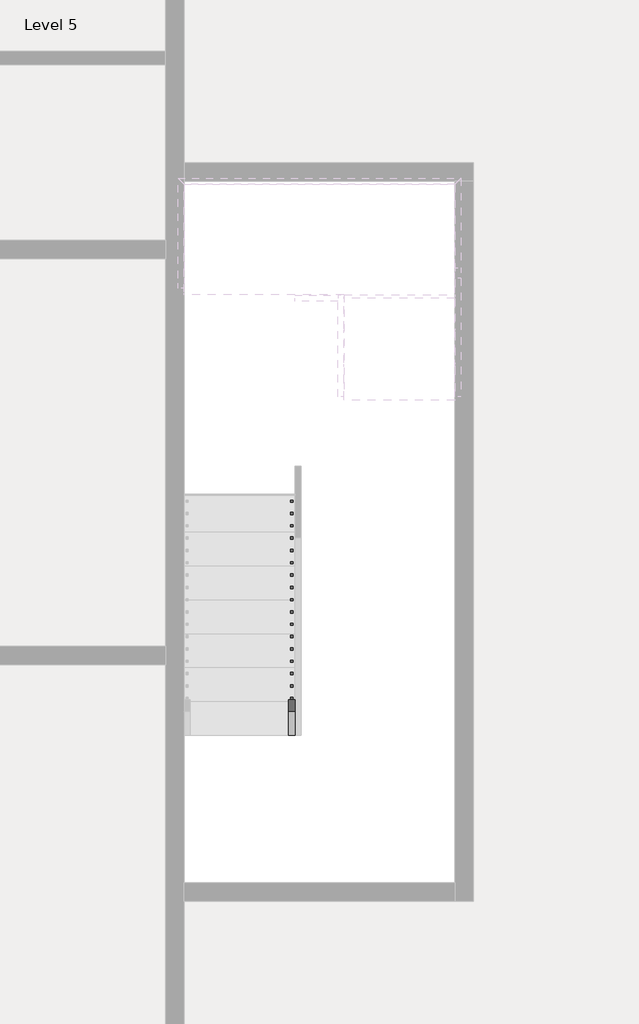
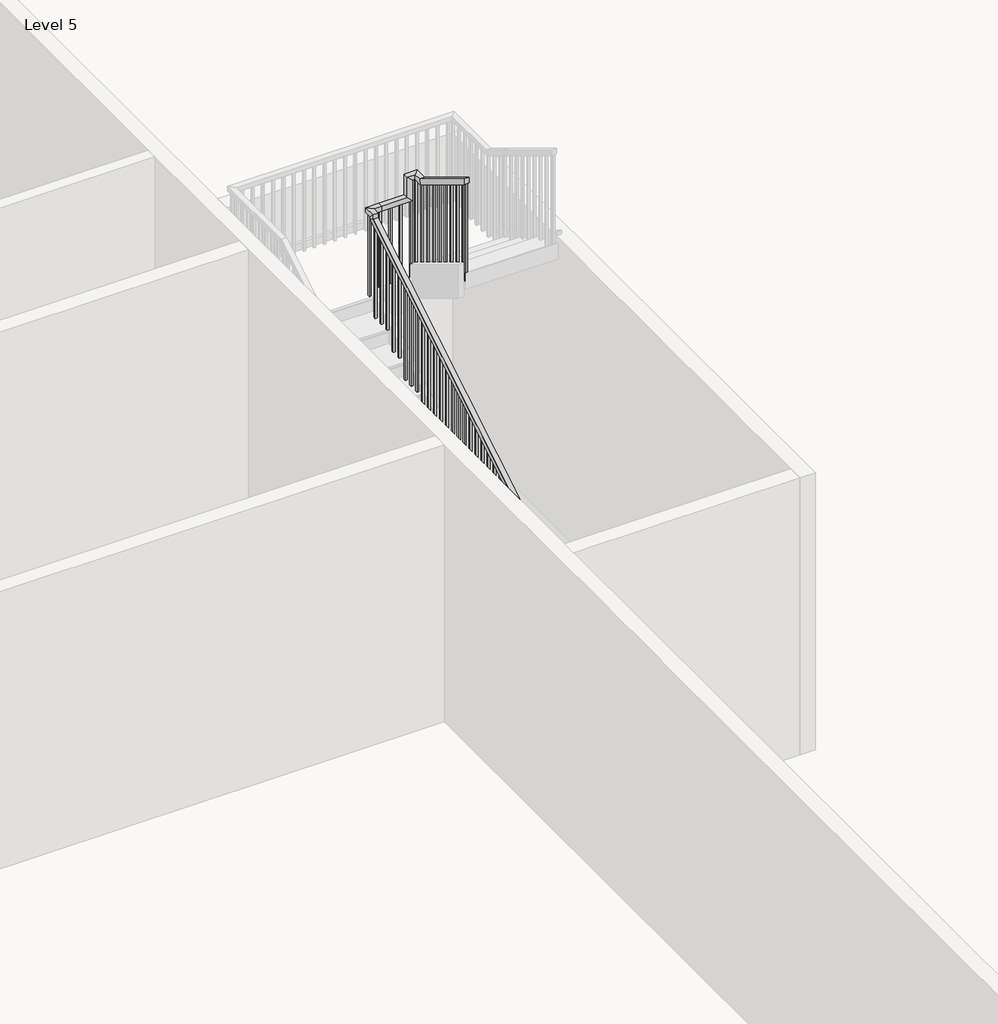
# One storey, part 5 of 8: 1 railing.
"""IFC4 building model written with IfcOpenShell, lengths in millimetres."""

from ifc_helpers import new_model, si_unit, frame, origin, place, context, project, spatial, polyline, outline, extrude, faceted_brep, element, save

model = new_model("IFC4")

# Units and contexts
model_context = context("Model", 3, world=origin())
ifc_project = project(units=[si_unit("LENGTHUNIT", "METRE", prefix="MILLI")], contexts=[model_context])

# Site, building, storey
site = spatial("IfcSite", under=ifc_project)
building = spatial("IfcBuilding", under=site)
storey = spatial("IfcBuildingStorey", under=building, Name="Level 5", Elevation=37426.6172466)

# Railing
placement = place(None, origin())
element("IfcRailing", 1, ObjectType="Handrail - Rectangular", at=placement, inside=storey, context=model_context, shape_type="SolidModel", body=[
    faceted_brep([(-2753.8415084, -23154.3851539, 38510.3505799), (-2753.8415084, -23154.3851539, 38450.9491197), (-2703.0415084, -23154.3851539, 38450.9491197), (-2703.0415084, -23154.3851539, 38510.3505799), (-2753.8415084, -19598.3851539, 40665.5020951), (-2753.8415084, -19547.5851539, 40636.8885136), (-2703.0415084, -19547.5851539, 40636.8885136), (-2703.0415084, -19598.3851539, 40665.5020951), (-2753.8415084, -19598.3851539, 40711.6839133), (-2753.8415084, -19547.5851539, 40660.8839133), (-2703.0415084, -19547.5851539, 40660.8839133), (-2703.0415084, -19598.3851539, 40711.6839133), (-2753.8415084, -19471.3851539, 40711.6839133), (-2753.8415084, -19471.3851539, 40660.8839133), (-2703.0415084, -19522.1851539, 40660.8839133), (-2703.0415084, -19522.1851539, 40711.6839133), (-2626.8415084, -19471.3851539, 40711.6839133), (-2626.8415084, -19471.3851539, 40660.8839133), (-2626.8415084, -19522.1851539, 40660.8839133), (-2626.8415084, -19522.1851539, 40711.6839133), (-2372.8415084, -19471.3851539, 40711.6839133), (-2322.0415084, -19471.3851539, 40660.8839133), (-2322.0415084, -19522.1851539, 40660.8839133), (-2372.8415084, -19522.1851539, 40711.6839133), (-2372.8415084, -19471.3851539, 40927.1990648), (-2322.0415084, -19471.3851539, 40876.3990648), (-2322.0415084, -19522.1851539, 40876.3990648), (-2372.8415084, -19522.1851539, 40927.1990648), (-2245.8415084, -19471.3851539, 40927.1990648), (-2245.8415084, -19471.3851539, 40876.3990648), (-2296.6415084, -19522.1851539, 40876.3990648), (-2296.6415084, -19522.1851539, 40927.1990648), (-2245.8415084, -19598.3851539, 40927.1990648), (-2245.8415084, -19612.5775633, 40876.3990648), (-2296.6415084, -19612.5775633, 40876.3990648), (-2296.6415084, -19598.3851539, 40927.1990648), (-2245.8415084, -20360.3851539, 41389.0172466), (-2296.6415084, -20360.3851539, 41389.0172466), (-2296.6415084, -20360.3851539, 41329.6157863), (-2245.8415084, -20360.3851539, 41329.6157863)], [[[0, 1, 2, 3]], [[1, 0, 4, 5]], [[2, 1, 5, 6]], [[3, 2, 6, 7]], [[0, 3, 7, 4]], [[5, 4, 8, 9]], [[6, 5, 9, 10]], [[7, 6, 10, 11]], [[4, 7, 11, 8]], [[9, 8, 12, 13]], [[10, 9, 13, 14]], [[11, 10, 14, 15]], [[8, 11, 15, 12]], [[13, 12, 16, 17]], [[14, 13, 17, 18]], [[15, 14, 18, 19]], [[12, 15, 19, 16]], [[17, 16, 20, 21]], [[18, 17, 21, 22]], [[19, 18, 22, 23]], [[16, 19, 23, 20]], [[21, 20, 24, 25]], [[22, 21, 25, 26]], [[23, 22, 26, 27]], [[20, 23, 27, 24]], [[25, 24, 28, 29]], [[26, 25, 29, 30]], [[27, 26, 30, 31]], [[24, 27, 31, 28]], [[29, 28, 32, 33]], [[30, 29, 33, 34]], [[31, 30, 34, 35]], [[28, 31, 35, 32]], [[36, 37, 38, 39]], [[33, 32, 36, 39]], [[34, 33, 39, 38]], [[35, 34, 38, 37]], [[32, 35, 37, 36]]]),
    extrude(outline(polyline([(-20319.1101539, 41304.6006348), (-20300.0601539, 41293.0551803), (-20300.0601539, 40305.2839133), (-20319.1101539, 40305.2839133), (-20319.1101539, 41304.6006348)])), frame((-2280.7665084, 0.0, 0.0), z_axis=(1.0, 0.0, 0.0), x_axis=(0.0, 1.0, 0.0)), (0.0, 0.0, 1.0), 19.05),
    extrude(outline(polyline([(-20217.5101539, 41243.0248773), (-20198.4601539, 41231.4794227), (-20198.4601539, 40305.2839133), (-20217.5101539, 40305.2839133), (-20217.5101539, 41243.0248773)])), frame((-2280.7665084, 0.0, 0.0), z_axis=(1.0, 0.0, 0.0), x_axis=(0.0, 1.0, 0.0)), (0.0, 0.0, 1.0), 19.05),
    extrude(outline(polyline([(-20115.9101539, 41181.4491197), (-20096.8601539, 41169.9036651), (-20096.8601539, 40305.2839133), (-20115.9101539, 40305.2839133), (-20115.9101539, 41181.4491197)])), frame((-2280.7665084, 0.0, 0.0), z_axis=(1.0, 0.0, 0.0), x_axis=(0.0, 1.0, 0.0)), (0.0, 0.0, 1.0), 19.05),
    extrude(outline(polyline([(-20014.3101539, 41119.8733621), (-19995.2601539, 41108.3279076), (-19995.2601539, 40135.9505799), (-20014.3101539, 40135.9505799), (-20014.3101539, 41119.8733621)])), frame((-2280.7665084, 0.0, 0.0), z_axis=(1.0, 0.0, 0.0), x_axis=(0.0, 1.0, 0.0)), (0.0, 0.0, 1.0), 19.05),
    extrude(outline(polyline([(-19912.7101539, 41058.2976045), (-19893.6601539, 41046.75215), (-19893.6601539, 40135.9505799), (-19912.7101539, 40135.9505799), (-19912.7101539, 41058.2976045)])), frame((-2280.7665084, 0.0, 0.0), z_axis=(1.0, 0.0, 0.0), x_axis=(0.0, 1.0, 0.0)), (0.0, 0.0, 1.0), 19.05),
    extrude(outline(polyline([(-19811.1101539, 40996.721847), (-19792.0601539, 40985.1763924), (-19792.0601539, 40135.9505799), (-19811.1101539, 40135.9505799), (-19811.1101539, 40996.721847)])), frame((-2280.7665084, 0.0, 0.0), z_axis=(1.0, 0.0, 0.0), x_axis=(0.0, 1.0, 0.0)), (0.0, 0.0, 1.0), 19.05),
    extrude(outline(polyline([(-19709.5101539, 40935.1460894), (-19690.4601539, 40923.6006348), (-19690.4601539, 39966.6172466), (-19709.5101539, 39966.6172466), (-19709.5101539, 40935.1460894)])), frame((-2280.7665084, 0.0, 0.0), z_axis=(1.0, 0.0, 0.0), x_axis=(0.0, 1.0, 0.0)), (0.0, 0.0, 1.0), 19.05),
    extrude(outline(polyline([(-19607.9101539, 40873.5703318), (-19588.8601539, 40862.0248773), (-19588.8601539, 39966.6172466), (-19607.9101539, 39966.6172466), (-19607.9101539, 40873.5703318)])), frame((-2280.7665084, 0.0, 0.0), z_axis=(1.0, 0.0, 0.0), x_axis=(0.0, 1.0, 0.0)), (0.0, 0.0, 1.0), 19.05),
    extrude(outline(polyline([(-2331.5665084, -19506.3101539), (-2331.5665084, -19487.2601539), (-2312.5165084, -19487.2601539), (-2312.5165084, -19506.3101539), (-2331.5665084, -19506.3101539)])), frame((0.0, 0.0, 39797.2839133), z_axis=(0.0, 0.0, 1.0), x_axis=(1.0, 0.0, 0.0)), (0.0, 0.0, 1.0), 1079.1151515),
    extrude(outline(polyline([(-2433.1665084, -19506.3101539), (-2433.1665084, -19487.2601539), (-2414.1165084, -19487.2601539), (-2414.1165084, -19506.3101539), (-2433.1665084, -19506.3101539)])), frame((0.0, 0.0, 39797.2839133), z_axis=(0.0, 0.0, 1.0), x_axis=(1.0, 0.0, 0.0)), (0.0, 0.0, 1.0), 863.6),
    extrude(outline(polyline([(-2534.7665084, -19506.3101539), (-2534.7665084, -19487.2601539), (-2515.7165084, -19487.2601539), (-2515.7165084, -19506.3101539), (-2534.7665084, -19506.3101539)])), frame((0.0, 0.0, 39797.2839133), z_axis=(0.0, 0.0, 1.0), x_axis=(1.0, 0.0, 0.0)), (0.0, 0.0, 1.0), 863.6),
    extrude(outline(polyline([(-2636.3665084, -19506.3101539), (-2636.3665084, -19487.2601539), (-2617.3165084, -19487.2601539), (-2617.3165084, -19506.3101539), (-2636.3665084, -19506.3101539)])), frame((0.0, 0.0, 39797.2839133), z_axis=(0.0, 0.0, 1.0), x_axis=(1.0, 0.0, 0.0)), (0.0, 0.0, 1.0), 863.6),
    extrude(outline(polyline([(-19607.9101539, 40600.3279076), (-19588.8601539, 40611.8733621), (-19588.8601539, 39627.9505799), (-19607.9101539, 39627.9505799), (-19607.9101539, 40600.3279076)])), frame((-2737.9665084, 0.0, 0.0), z_axis=(1.0, 0.0, 0.0), x_axis=(0.0, 1.0, 0.0)), (0.0, 0.0, 1.0), 19.05),
    extrude(outline(polyline([(-19709.5101539, 40538.75215), (-19690.4601539, 40550.2976045), (-19690.4601539, 39627.9505799), (-19709.5101539, 39627.9505799), (-19709.5101539, 40538.75215)])), frame((-2737.9665084, 0.0, 0.0), z_axis=(1.0, 0.0, 0.0), x_axis=(0.0, 1.0, 0.0)), (0.0, 0.0, 1.0), 19.05),
    extrude(outline(polyline([(-19811.1101539, 40477.1763924), (-19792.0601539, 40488.721847), (-19792.0601539, 39627.9505799), (-19811.1101539, 39627.9505799), (-19811.1101539, 40477.1763924)])), frame((-2737.9665084, 0.0, 0.0), z_axis=(1.0, 0.0, 0.0), x_axis=(0.0, 1.0, 0.0)), (0.0, 0.0, 1.0), 19.05),
    extrude(outline(polyline([(-19912.7101539, 40415.6006348), (-19893.6601539, 40427.1460894), (-19893.6601539, 39458.6172466), (-19912.7101539, 39458.6172466), (-19912.7101539, 40415.6006348)])), frame((-2737.9665084, 0.0, 0.0), z_axis=(1.0, 0.0, 0.0), x_axis=(0.0, 1.0, 0.0)), (0.0, 0.0, 1.0), 19.05),
    extrude(outline(polyline([(-20014.3101539, 40354.0248773), (-19995.2601539, 40365.5703318), (-19995.2601539, 39458.6172466), (-20014.3101539, 39458.6172466), (-20014.3101539, 40354.0248773)])), frame((-2737.9665084, 0.0, 0.0), z_axis=(1.0, 0.0, 0.0), x_axis=(0.0, 1.0, 0.0)), (0.0, 0.0, 1.0), 19.05),
    extrude(outline(polyline([(-20115.9101539, 40292.4491197), (-20096.8601539, 40303.9945742), (-20096.8601539, 39289.2839133), (-20115.9101539, 39289.2839133), (-20115.9101539, 40292.4491197)])), frame((-2737.9665084, 0.0, 0.0), z_axis=(1.0, 0.0, 0.0), x_axis=(0.0, 1.0, 0.0)), (0.0, 0.0, 1.0), 19.05),
    extrude(outline(polyline([(-20217.5101539, 40230.8733621), (-20198.4601539, 40242.4188166), (-20198.4601539, 39289.2839133), (-20217.5101539, 39289.2839133), (-20217.5101539, 40230.8733621)])), frame((-2737.9665084, 0.0, 0.0), z_axis=(1.0, 0.0, 0.0), x_axis=(0.0, 1.0, 0.0)), (0.0, 0.0, 1.0), 19.05),
    extrude(outline(polyline([(-20319.1101539, 40169.2976045), (-20300.0601539, 40180.8430591), (-20300.0601539, 39289.2839133), (-20319.1101539, 39289.2839133), (-20319.1101539, 40169.2976045)])), frame((-2737.9665084, 0.0, 0.0), z_axis=(1.0, 0.0, 0.0), x_axis=(0.0, 1.0, 0.0)), (0.0, 0.0, 1.0), 19.05),
    extrude(outline(polyline([(-20420.7101539, 40107.721847), (-20401.6601539, 40119.2673015), (-20401.6601539, 39119.9505799), (-20420.7101539, 39119.9505799), (-20420.7101539, 40107.721847)])), frame((-2737.9665084, 0.0, 0.0), z_axis=(1.0, 0.0, 0.0), x_axis=(0.0, 1.0, 0.0)), (0.0, 0.0, 1.0), 19.05),
    extrude(outline(polyline([(-20522.3101539, 40046.1460894), (-20503.2601539, 40057.6915439), (-20503.2601539, 39119.9505799), (-20522.3101539, 39119.9505799), (-20522.3101539, 40046.1460894)])), frame((-2737.9665084, 0.0, 0.0), z_axis=(1.0, 0.0, 0.0), x_axis=(0.0, 1.0, 0.0)), (0.0, 0.0, 1.0), 19.05),
    extrude(outline(polyline([(-20623.9101539, 39984.5703318), (-20604.8601539, 39996.1157863), (-20604.8601539, 39119.9505799), (-20623.9101539, 39119.9505799), (-20623.9101539, 39984.5703318)])), frame((-2737.9665084, 0.0, 0.0), z_axis=(1.0, 0.0, 0.0), x_axis=(0.0, 1.0, 0.0)), (0.0, 0.0, 1.0), 19.05),
    extrude(outline(polyline([(-20725.5101539, 39922.9945742), (-20706.4601539, 39934.5400288), (-20706.4601539, 38950.6172466), (-20725.5101539, 38950.6172466), (-20725.5101539, 39922.9945742)])), frame((-2737.9665084, 0.0, 0.0), z_axis=(1.0, 0.0, 0.0), x_axis=(0.0, 1.0, 0.0)), (0.0, 0.0, 1.0), 19.05),
    extrude(outline(polyline([(-20827.1101539, 39861.4188166), (-20808.0601539, 39872.9642712), (-20808.0601539, 38950.6172466), (-20827.1101539, 38950.6172466), (-20827.1101539, 39861.4188166)])), frame((-2737.9665084, 0.0, 0.0), z_axis=(1.0, 0.0, 0.0), x_axis=(0.0, 1.0, 0.0)), (0.0, 0.0, 1.0), 19.05),
    extrude(outline(polyline([(-20928.7101539, 39799.8430591), (-20909.6601539, 39811.3885136), (-20909.6601539, 38950.6172466), (-20928.7101539, 38950.6172466), (-20928.7101539, 39799.8430591)])), frame((-2737.9665084, 0.0, 0.0), z_axis=(1.0, 0.0, 0.0), x_axis=(0.0, 1.0, 0.0)), (0.0, 0.0, 1.0), 19.05),
    extrude(outline(polyline([(-21030.3101539, 39738.2673015), (-21011.2601539, 39749.812756), (-21011.2601539, 38781.2839133), (-21030.3101539, 38781.2839133), (-21030.3101539, 39738.2673015)])), frame((-2737.9665084, 0.0, 0.0), z_axis=(1.0, 0.0, 0.0), x_axis=(0.0, 1.0, 0.0)), (0.0, 0.0, 1.0), 19.05),
    extrude(outline(polyline([(-21131.9101539, 39676.6915439), (-21112.8601539, 39688.2369985), (-21112.8601539, 38781.2839133), (-21131.9101539, 38781.2839133), (-21131.9101539, 39676.6915439)])), frame((-2737.9665084, 0.0, 0.0), z_axis=(1.0, 0.0, 0.0), x_axis=(0.0, 1.0, 0.0)), (0.0, 0.0, 1.0), 19.05),
    extrude(outline(polyline([(-21233.5101539, 39615.1157863), (-21214.4601539, 39626.6612409), (-21214.4601539, 38611.9505799), (-21233.5101539, 38611.9505799), (-21233.5101539, 39615.1157863)])), frame((-2737.9665084, 0.0, 0.0), z_axis=(1.0, 0.0, 0.0), x_axis=(0.0, 1.0, 0.0)), (0.0, 0.0, 1.0), 19.05),
    extrude(outline(polyline([(-21335.1101539, 39553.5400288), (-21316.0601539, 39565.0854833), (-21316.0601539, 38611.9505799), (-21335.1101539, 38611.9505799), (-21335.1101539, 39553.5400288)])), frame((-2737.9665084, 0.0, 0.0), z_axis=(1.0, 0.0, 0.0), x_axis=(0.0, 1.0, 0.0)), (0.0, 0.0, 1.0), 19.05),
    extrude(outline(polyline([(-21436.7101539, 39491.9642712), (-21417.6601539, 39503.5097257), (-21417.6601539, 38611.9505799), (-21436.7101539, 38611.9505799), (-21436.7101539, 39491.9642712)])), frame((-2737.9665084, 0.0, 0.0), z_axis=(1.0, 0.0, 0.0), x_axis=(0.0, 1.0, 0.0)), (0.0, 0.0, 1.0), 19.05),
    extrude(outline(polyline([(-21538.3101539, 39430.3885136), (-21519.2601539, 39441.9339682), (-21519.2601539, 38442.6172466), (-21538.3101539, 38442.6172466), (-21538.3101539, 39430.3885136)])), frame((-2737.9665084, 0.0, 0.0), z_axis=(1.0, 0.0, 0.0), x_axis=(0.0, 1.0, 0.0)), (0.0, 0.0, 1.0), 19.05),
    extrude(outline(polyline([(-21639.9101539, 39368.812756), (-21620.8601539, 39380.3582106), (-21620.8601539, 38442.6172466), (-21639.9101539, 38442.6172466), (-21639.9101539, 39368.812756)])), frame((-2737.9665084, 0.0, 0.0), z_axis=(1.0, 0.0, 0.0), x_axis=(0.0, 1.0, 0.0)), (0.0, 0.0, 1.0), 19.05),
    extrude(outline(polyline([(-21741.5101539, 39307.2369985), (-21722.4601539, 39318.782453), (-21722.4601539, 38442.6172466), (-21741.5101539, 38442.6172466), (-21741.5101539, 39307.2369985)])), frame((-2737.9665084, 0.0, 0.0), z_axis=(1.0, 0.0, 0.0), x_axis=(0.0, 1.0, 0.0)), (0.0, 0.0, 1.0), 19.05),
    extrude(outline(polyline([(-21843.1101539, 39245.6612409), (-21824.0601539, 39257.2066954), (-21824.0601539, 38273.2839133), (-21843.1101539, 38273.2839133), (-21843.1101539, 39245.6612409)])), frame((-2737.9665084, 0.0, 0.0), z_axis=(1.0, 0.0, 0.0), x_axis=(0.0, 1.0, 0.0)), (0.0, 0.0, 1.0), 19.05),
    extrude(outline(polyline([(-21944.7101539, 39184.0854833), (-21925.6601539, 39195.6309379), (-21925.6601539, 38273.2839133), (-21944.7101539, 38273.2839133), (-21944.7101539, 39184.0854833)])), frame((-2737.9665084, 0.0, 0.0), z_axis=(1.0, 0.0, 0.0), x_axis=(0.0, 1.0, 0.0)), (0.0, 0.0, 1.0), 19.05),
    extrude(outline(polyline([(-22046.3101539, 39122.5097257), (-22027.2601539, 39134.0551803), (-22027.2601539, 38273.2839133), (-22046.3101539, 38273.2839133), (-22046.3101539, 39122.5097257)])), frame((-2737.9665084, 0.0, 0.0), z_axis=(1.0, 0.0, 0.0), x_axis=(0.0, 1.0, 0.0)), (0.0, 0.0, 1.0), 19.05),
    extrude(outline(polyline([(-22147.9101539, 39060.9339682), (-22128.8601539, 39072.4794227), (-22128.8601539, 38103.9505799), (-22147.9101539, 38103.9505799), (-22147.9101539, 39060.9339682)])), frame((-2737.9665084, 0.0, 0.0), z_axis=(1.0, 0.0, 0.0), x_axis=(0.0, 1.0, 0.0)), (0.0, 0.0, 1.0), 19.05),
    extrude(outline(polyline([(-22249.5101539, 38999.3582106), (-22230.4601539, 39010.9036651), (-22230.4601539, 38103.9505799), (-22249.5101539, 38103.9505799), (-22249.5101539, 38999.3582106)])), frame((-2737.9665084, 0.0, 0.0), z_axis=(1.0, 0.0, 0.0), x_axis=(0.0, 1.0, 0.0)), (0.0, 0.0, 1.0), 19.05),
    extrude(outline(polyline([(-22351.1101539, 38937.782453), (-22332.0601539, 38949.3279076), (-22332.0601539, 37934.6172466), (-22351.1101539, 37934.6172466), (-22351.1101539, 38937.782453)])), frame((-2737.9665084, 0.0, 0.0), z_axis=(1.0, 0.0, 0.0), x_axis=(0.0, 1.0, 0.0)), (0.0, 0.0, 1.0), 19.05),
    extrude(outline(polyline([(-22452.7101539, 38876.2066954), (-22433.6601539, 38887.75215), (-22433.6601539, 37934.6172466), (-22452.7101539, 37934.6172466), (-22452.7101539, 38876.2066954)])), frame((-2737.9665084, 0.0, 0.0), z_axis=(1.0, 0.0, 0.0), x_axis=(0.0, 1.0, 0.0)), (0.0, 0.0, 1.0), 19.05),
    extrude(outline(polyline([(-22554.3101539, 38814.6309379), (-22535.2601539, 38826.1763924), (-22535.2601539, 37934.6172466), (-22554.3101539, 37934.6172466), (-22554.3101539, 38814.6309379)])), frame((-2737.9665084, 0.0, 0.0), z_axis=(1.0, 0.0, 0.0), x_axis=(0.0, 1.0, 0.0)), (0.0, 0.0, 1.0), 19.05),
    extrude(outline(polyline([(-22655.9101539, 38753.0551803), (-22636.8601539, 38764.6006348), (-22636.8601539, 37765.2839133), (-22655.9101539, 37765.2839133), (-22655.9101539, 38753.0551803)])), frame((-2737.9665084, 0.0, 0.0), z_axis=(1.0, 0.0, 0.0), x_axis=(0.0, 1.0, 0.0)), (0.0, 0.0, 1.0), 19.05),
    extrude(outline(polyline([(-22757.5101539, 38691.4794227), (-22738.4601539, 38703.0248773), (-22738.4601539, 37765.2839133), (-22757.5101539, 37765.2839133), (-22757.5101539, 38691.4794227)])), frame((-2737.9665084, 0.0, 0.0), z_axis=(1.0, 0.0, 0.0), x_axis=(0.0, 1.0, 0.0)), (0.0, 0.0, 1.0), 19.05),
    extrude(outline(polyline([(-22859.1101539, 38629.9036651), (-22840.0601539, 38641.4491197), (-22840.0601539, 37765.2839133), (-22859.1101539, 37765.2839133), (-22859.1101539, 38629.9036651)])), frame((-2737.9665084, 0.0, 0.0), z_axis=(1.0, 0.0, 0.0), x_axis=(0.0, 1.0, 0.0)), (0.0, 0.0, 1.0), 19.05),
    extrude(outline(polyline([(-22960.7101539, 38568.3279076), (-22941.6601539, 38579.8733621), (-22941.6601539, 37595.9505799), (-22960.7101539, 37595.9505799), (-22960.7101539, 38568.3279076)])), frame((-2737.9665084, 0.0, 0.0), z_axis=(1.0, 0.0, 0.0), x_axis=(0.0, 1.0, 0.0)), (0.0, 0.0, 1.0), 19.05),
    extrude(outline(polyline([(-23062.3101539, 38506.75215), (-23043.2601539, 38518.2976045), (-23043.2601539, 37595.9505799), (-23062.3101539, 37595.9505799), (-23062.3101539, 38506.75215)])), frame((-2737.9665084, 0.0, 0.0), z_axis=(1.0, 0.0, 0.0), x_axis=(0.0, 1.0, 0.0)), (0.0, 0.0, 1.0), 19.05),
    extrude(outline(polyline([(-2280.7665084, -19506.3101539), (-2280.7665084, -19487.2601539), (-2261.7165084, -19487.2601539), (-2261.7165084, -19506.3101539), (-2280.7665084, -19506.3101539)])), frame((0.0, 0.0, 39797.2839133), z_axis=(0.0, 0.0, 1.0), x_axis=(1.0, 0.0, 0.0)), (0.0, 0.0, 1.0), 1079.1151515),
    extrude(outline(polyline([(-2718.9165084, -19506.3101539), (-2737.9665084, -19506.3101539), (-2737.9665084, -19487.2601539), (-2718.9165084, -19487.2601539), (-2718.9165084, -19506.3101539)])), frame((0.0, 0.0, 39797.2839133), z_axis=(0.0, 0.0, 1.0), x_axis=(1.0, 0.0, 0.0)), (0.0, 0.0, 1.0), 863.6),
    extrude(outline(polyline([(-20360.3851539, 41329.6157863), (-20341.3351539, 41318.0703318), (-20341.3351539, 40305.2839133), (-20360.3851539, 40305.2839133), (-20360.3851539, 41329.6157863)])), frame((-2280.7665084, 0.0, 0.0), z_axis=(1.0, 0.0, 0.0), x_axis=(0.0, 1.0, 0.0)), (0.0, 0.0, 1.0), 19.05),
    extrude(outline(polyline([(-23154.3851539, 38450.9491197), (-23135.3351539, 38462.4945742), (-23135.3351539, 37595.9505799), (-23154.3851539, 37595.9505799), (-23154.3851539, 38450.9491197)])), frame((-2737.9665084, 0.0, 0.0), z_axis=(1.0, 0.0, 0.0), x_axis=(0.0, 1.0, 0.0)), (0.0, 0.0, 1.0), 19.05),
])

save(model, "model.ifc")

# Revit data of these elements
# Type "Handrail - Rectangular"
#   Assembly Code = "C2010400"
#   built-in parameter 1008612 = 0.0416667 (stored number, unit not read)
#   built-in parameter 1008611 = 0.0416667 (stored number, unit not read)
#   built-in parameter 1008609 = 0.333333 (stored number, unit not read)
#   built-in parameter 1008604 = 0.166667 (stored number, unit not read)
#   built-in parameter 1008603 = 0.166667 (stored number, unit not read)
#   Railing Height = 3' - 0"
#   built-in parameter 1008630 = 2
#   built-in parameter 1008610 = 2
#   built-in parameter 1008618 = Baluster - Square : 3/4"
# Element 1 (IfcRailing, "Handrail - Rectangular")
#   Phase Created = New Construction
